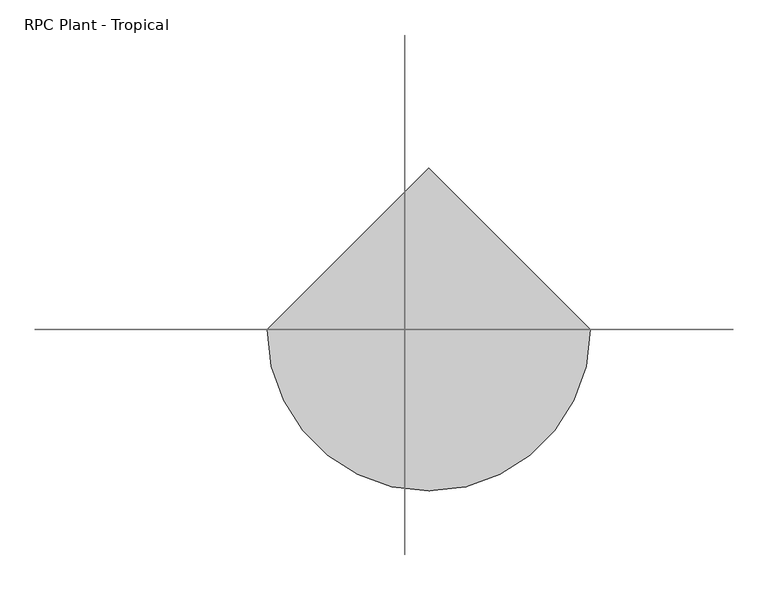
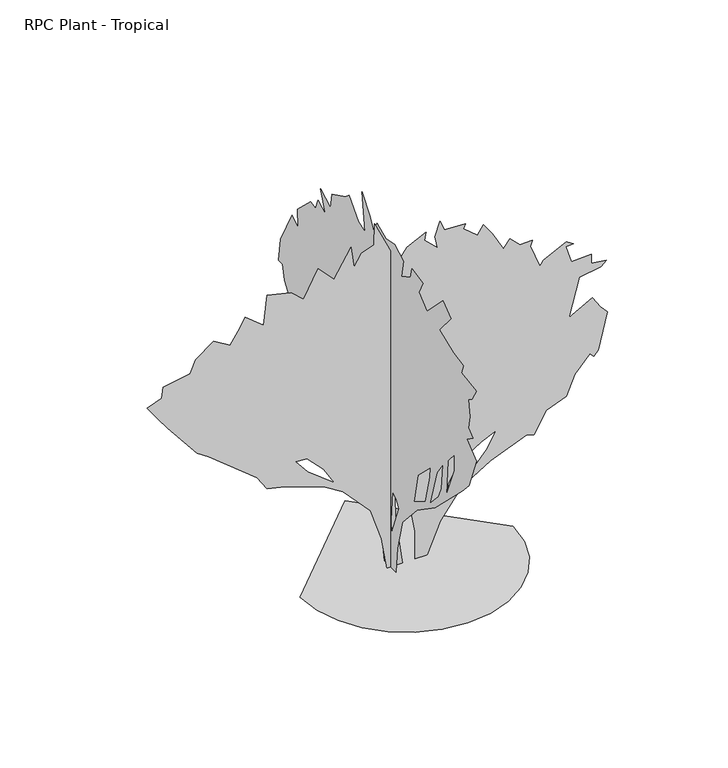
"""IFC4 building model written with IfcOpenShell, lengths in millimetres: geographic element geometry, RPC Plant - Tropical."""

from ifc_helpers import new_model, si_unit, origin, place, context, project, spatial, triangles, source, transform, mapped, element, save


def rpc_plant_tropical_6475341c(model_context):
    return source(origin(), model_context, "Body", "Tessellation", [
        triangles([(-396.3767504, 0.0, 8.22e-05), (-385.8992649, -90.8237077, 8.22e-05), (-356.0543206, -174.2306261, 8.22e-05), (-309.2370838, -247.8313661, 8.22e-05), (-247.8313661, -309.2370838, 8.22e-05), (-174.2306261, -356.0543206, 8.22e-05), (-90.8237077, -385.8992649, 8.22e-05), (1.73e-05, -396.3767504, 8.22e-05), (90.8237077, -385.8992649, 8.22e-05), (174.2306261, -356.0543206, 8.22e-05), (247.8313661, -309.2370838, 8.22e-05), (309.2370838, -247.8313661, 8.22e-05), (356.0543206, -174.2306261, 8.22e-05), (385.8992649, -90.8237077, 8.22e-05), (396.3767504, 3.47e-05, 8.22e-05), (-5.2e-05, 396.3767504, 8.22e-05), (-59.3577095, -35.0059915, 9.26e-05), (-59.3577095, -44.8705806, 101.5460546), (-59.3577095, -75.4742449, 222.0478563), (-59.3577095, -168.9964434, 326.3007588), (-59.3577095, -285.8741748, 405.6706235), (-59.3579639, -459.2340692, 576.3228888), (-59.3579639, -503.9253456, 625.6344137), (-59.3579639, -553.1479589, 751.1941189), (-59.3579639, -491.6190474, 799.7715317), (-59.3579639, -530.478485, 828.915465), (-59.3579639, -501.3320083, 851.5849388), (-59.3579639, -511.0474763, 900.1598808), (-59.3579639, -501.3320083, 961.688756), (-59.3579639, -524.0014821, 977.8812269), (-59.3579639, -553.1479589, 1026.4561689), (-59.3579639, -455.9955677, 1039.4101748), (-59.3579639, -469.4956884, 1077.0376745), (-59.3579639, -404.1821606, 1087.9850441), (-59.3579639, -313.5068087, 1123.6085238), (-59.3579639, -387.9896896, 1211.0454105), (-59.3579639, -336.1762825, 1249.9048119), (-59.3579639, -235.7859349, 1149.5164627), (-59.3579639, -183.9712561, 1191.6144018), (-59.3579639, -209.8784683, 1243.4278816), (-59.3579639, -138.9198272, 1256.3183739), (-59.3579639, -128.9188388, 1217.5224134), (-59.3579639, -70.6279291, 1185.1373989), (-59.3579639, -83.5816624, 1253.143277), (-59.3579639, -25.4436618, 1284.1769932), (-59.3579639, 29.761912, 1272.5743584), (-59.3579639, 86.0073592, 1299.3586246), (-59.3579639, 110.7212849, 1256.3817421), (-59.3579639, 133.3899957, 1298.4822247), (-59.3579639, 185.2039207, 1363.2496376), (-59.3577095, 165.7739475, 1217.5224134), (-59.3577095, 207.8728858, 1230.4738758), (-59.3577095, 266.3644464, 1299.9199276), (-59.3577095, 292.0717617, 1279.0512886), (-59.3577095, 376.2676217, 1236.950806), (-59.3577095, 385.9830897, 1178.660396), (-59.3577095, 450.7505027, 1214.2838757), (-59.3577095, 418.3680679, 1133.3239918), (-59.3577095, 466.9429736, 1159.22946), (-59.3577095, 484.2835213, 1117.1086298), (-59.3577095, 515.5204227, 1123.6085238), (-59.3577095, 599.7162646, 1042.6486399), (-59.3577095, 596.4777632, 974.6427618), (-59.3577095, 635.3397079, 997.3122356), (-59.3577095, 709.8225889, 858.0619417), (-59.3577095, 722.7765947, 767.3865898), (-59.3577095, 696.8686558, 767.3865898), (-59.3577095, 683.91465, 712.3346449), (-59.3577095, 619.147237, 621.659293), (-59.3577095, 586.7622588, 628.1362959), (-59.3577095, 577.0493342, 595.7513177), (-59.3577095, 544.664356, 589.2743148), (-59.3577095, 512.2819213, 514.7914338), (-59.3577095, 453.9890041, 501.8400078), (-59.3577095, 473.4199765, 479.1705339), (-59.3577095, 438.083507, 433.2245012), (-59.3577095, 424.8450708, 430.5955919), (-59.3577095, 359.671251, 388.3935531), (-59.3577095, 230.5626891, 332.9860339), (-59.3577095, 112.6590482, 224.7923109), (-59.3577095, 55.1474106, 87.2636415), (-59.3577095, 39.476642, 8.38e-05), (-59.3577095, -5.8605105, 135.9018064), (-59.3577095, -2.7896791, 186.1833303), (-59.3577095, -12.337225, 304.2967785), (-59.3577095, -38.2442317, 288.1068329), (-59.3577095, -54.4362076, 262.1988576), (-59.3577095, -151.5875587, 349.6357444), (-59.3577095, -177.4947618, 469.4550296), (-59.3577095, -258.4549001, 547.176412), (-59.3577095, -255.2163986, 508.3169744), (-59.3577095, -226.0704487, 394.9721486), (-59.3577095, -255.2163986, 404.687653), (-59.3577095, -297.3143196, 550.4149135), (-59.3577095, -337.517407, 606.5056758), (-59.3577095, -326.4607781, 505.0785092), (-59.3577095, -307.0298058, 462.9780267), (-59.3577095, -358.8432129, 501.8400078), (-59.3579639, -368.5587173, 641.0903017), (-59.3579639, -410.6591635, 689.6651711), (-59.3579639, -410.6591635, 628.1362959), (-59.3577095, 198.157654, 356.112711), (-59.3577095, 261.769596, 391.7057055), (-59.3577095, 324.4541782, 475.9320325), (-59.3577095, 282.3562755, 469.4550296), (-59.3577095, 253.2100531, 430.5955919), (-267.2940953, 2.61e-05, 404.687653), (-308.6096875, 2.21e-05, 471.3142911), (-370.9208914, 1.84e-05, 534.2224425), (-413.0213739, 1.82e-05, 537.4609076), (-368.4215527, 2.15e-05, 482.1804156), (30.6369404, 5.02e-05, 0.0), (31.1304627, 4.38e-05, 108.1619844), (9.0696959, 3.61e-05, 237.4841779), (-47.0839311, 3.05e-05, 330.2047357), (-39.4309189, 4.01e-05, 170.4041154), (-14.7000316, 5.02e-05, 0.0), (-72.990889, 5.02e-05, 0.0), (-92.9872747, 4.29e-05, 122.5858678), (-134.4006626, 3.55e-05, 247.1552083), (-236.0793036, 2.88e-05, 358.7517941), (-302.2063538, 2.64e-05, 398.8659516), (-451.8807753, 2.32e-05, 453.2625587), (-519.8892331, 2.22e-05, 469.4550296), (-555.510133, 1.89e-05, 524.5069382), (-736.858366, 1.03e-05, 670.234235), (-778.9587759, 8.5e-06, 699.3807117), (-889.0625931, 4e-07, 835.3924679), (-924.6860727, -2.5e-06, 883.9674099), (-965.6003632, -6e-06, 942.4685629), (-911.7320669, -7.1e-06, 961.688756), (-905.255064, -9.6e-06, 1003.7892385), (-804.8642441, -1.06e-05, 1019.979166), (-785.4357788, -1.35e-05, 1068.5565788), (-717.4299007, -1.64e-05, 1117.1315208), (-655.8984821, -1.43e-05, 1081.5105846), (-620.2775459, -1.75e-05, 1136.5625296), (-600.8465735, -1.97e-05, 1172.1833931), (-532.8406591, -1.64e-05, 1117.1315208), (-519.8892331, -2.31e-05, 1230.4738758), (-429.2138449, -2.18e-05, 1207.8068727), (-383.8748972, -1.93e-05, 1165.7064629), (-328.8229886, -2.53e-05, 1266.0972828), (-270.5325967, -2.16e-05, 1204.5684076), (-205.7644389, -2.78e-05, 1308.1951492), (-196.0496976, -2.29e-05, 1227.2378815), (-167.6639666, -2.55e-05, 1270.8241745), (-121.5665623, -2.66e-05, 1288.7668293), (-119.7654549, -3.15e-05, 1371.5986919), (-34.1304544, -2.06e-05, 1188.3759367), (2.3015577, -2.34e-05, 1235.4267712), (72.7363851, -2.54e-05, 1269.3357479), (66.2596456, -2.37e-05, 1240.1892712), (114.8353143, -2.1e-05, 1194.8529396), (105.1200825, -2.37e-05, 1240.1892712), (124.5505553, -2.7e-05, 1295.2437595), (140.7425266, -2.47e-05, 1256.3817421), (218.4636638, -2.45e-05, 1253.143277), (211.1367854, -2.35e-05, 1235.7950626), (263.8015941, -2.08e-05, 1191.6144018), (286.4685245, -2.27e-05, 1223.9994164), (318.8535027, -2e-05, 1178.660396), (360.9514054, -1.56e-05, 1104.177515), (385.0814006, -1.75e-05, 1135.7446289), (422.4828604, -1.52e-05, 1097.7005121), (467.8192646, -1.54e-05, 1100.9390499), (461.3422617, -1.41e-05, 1078.2721195), (496.9657413, -8.7e-06, 987.5967676), (509.9172037, -9.8e-06, 1007.0277037), (594.1155527, -1.23e-05, 1049.1256428), (620.0235643, -1.14e-05, 1032.9331718), (593.290058, -1.13e-05, 1031.1069025), (613.5465614, -7.3e-06, 964.9272211), (688.0294424, -7.5e-06, 968.1657589), (688.0294424, -5.4e-06, 932.5448227), (743.0813147, -5e-06, 926.0678198), (723.6503786, -3.8e-06, 906.6368837), (642.6904947, -3.1e-06, 893.6828779), (603.8310571, 5.6e-06, 747.9555811), (691.2679075, 2.7e-06, 796.5330666), (720.4118408, 5.4e-06, 751.1941189), (746.3198524, 7.2e-06, 722.0501856), (713.9348379, 1.55e-05, 582.7973482), (697.7449104, 1.66e-05, 563.3688829), (681.5524395, 1.57e-05, 579.5613902), (626.5005672, 1.93e-05, 518.0299353), (594.1155527, 2.38e-05, 443.5470543), (519.6326717, 2.55e-05, 414.403121), (474.2962675, 3.03e-05, 333.4432371), (448.3882922, 2.98e-05, 343.1587415), (311.7719945, 3.3e-05, 288.0331637), (205.1723602, 3.7e-05, 221.2502851), (125.3034072, 4.32e-05, 117.1220752), (75.9746277, 5.02e-05, 0.0), (30.6369404, 3.34e-05, 281.62983), (43.5909303, 2.72e-05, 385.2566442), (7.9686832, 2.28e-05, 459.7395252), (-30.8919575, 2.45e-05, 430.5955919), (-38.6976243, 2.72e-05, 386.112624), (-2.6646859, 3.14e-05, 315.8842435), (150.4575132, 3.75e-05, 213.6229345), (215.0437962, 3.57e-05, 242.9182394), (296.5269221, 3.01e-05, 337.5199505), (331.8074721, 2.65e-05, 398.2106501), (278.0814637, 2.79e-05, 375.0661689), (195.3344433, 3.11e-05, 320.3901821), (154.7673882, 3.52e-05, 251.8887493)], [[15, 16, 1], [14, 15, 1], [14, 1, 2], [13, 14, 2], [13, 2, 3], [13, 3, 4], [12, 13, 4], [11, 12, 4], [11, 4, 5], [11, 5, 6], [11, 6, 7], [11, 7, 8], [11, 8, 9], [11, 9, 10], [93, 90, 91], [93, 91, 92], [90, 93, 94], [95, 98, 99], [83, 17, 18], [98, 95, 96], [49, 50, 51], [56, 57, 58], [88, 85, 86], [48, 49, 51], [102, 84, 85], [83, 18, 19], [87, 83, 19], [30, 31, 32], [87, 19, 20], [39, 40, 41], [39, 41, 42], [25, 26, 27], [29, 30, 32], [82, 17, 83], [81, 82, 83], [80, 81, 83], [80, 83, 84], [80, 84, 102], [79, 80, 102], [79, 102, 103], [78, 79, 103], [78, 103, 104], [77, 78, 104], [32, 33, 34], [65, 66, 67], [58, 59, 60], [35, 36, 37], [35, 37, 38], [88, 86, 87], [88, 87, 20], [92, 88, 20], [92, 20, 21], [93, 92, 21], [97, 93, 21], [97, 21, 22], [63, 64, 65], [52, 53, 54], [46, 47, 48], [74, 75, 76], [23, 24, 25], [43, 44, 45], [43, 45, 46], [98, 96, 97], [98, 97, 22], [101, 98, 22], [101, 22, 23], [101, 23, 25], [100, 101, 25], [68, 69, 70], [74, 76, 77], [74, 77, 104], [70, 71, 72], [85, 88, 89], [102, 85, 89], [106, 102, 89], [105, 106, 89], [52, 54, 55], [52, 55, 56], [60, 61, 62], [60, 62, 63], [39, 42, 43], [72, 73, 74], [43, 46, 48], [43, 48, 51], [63, 65, 67], [90, 94, 95], [105, 89, 90], [38, 39, 43], [63, 67, 68], [63, 68, 70], [63, 70, 72], [60, 63, 72], [58, 60, 72], [58, 72, 74], [58, 74, 104], [58, 104, 105], [58, 105, 90], [56, 58, 90], [52, 56, 90], [51, 52, 90], [43, 51, 90], [38, 43, 90], [38, 90, 95], [38, 95, 99], [38, 99, 100], [35, 38, 100], [35, 100, 25], [35, 25, 27], [34, 35, 27], [32, 34, 27], [29, 32, 27], [28, 29, 27], [196, 112, 113], [196, 197, 201], [195, 196, 113], [195, 113, 114], [148, 149, 150], [112, 196, 201], [170, 171, 172], [207, 201, 197], [144, 145, 146], [155, 156, 157], [175, 176, 177], [175, 177, 178], [151, 152, 153], [194, 112, 201], [193, 194, 201], [192, 193, 201], [192, 201, 202], [191, 192, 202], [191, 202, 203], [195, 114, 115], [200, 195, 115], [199, 200, 115], [169, 170, 172], [206, 207, 197], [157, 158, 159], [165, 166, 167], [160, 161, 162], [142, 143, 144], [129, 130, 131], [116, 117, 118], [116, 118, 119], [116, 119, 120], [115, 116, 120], [107, 115, 120], [107, 120, 121], [107, 121, 122], [111, 107, 122], [111, 122, 123], [110, 111, 123], [137, 138, 139], [199, 115, 107], [163, 164, 165], [139, 140, 141], [183, 184, 185], [190, 191, 203], [190, 203, 204], [173, 174, 175], [173, 175, 178], [169, 172, 173], [179, 180, 181], [198, 199, 107], [139, 141, 142], [188, 189, 190], [110, 123, 124], [110, 124, 125], [168, 169, 173], [154, 155, 157], [154, 157, 159], [131, 132, 133], [182, 183, 185], [188, 190, 204], [147, 148, 150], [146, 147, 150], [205, 206, 197], [136, 137, 139], [181, 182, 185], [179, 181, 185], [179, 185, 186], [134, 135, 136], [198, 107, 108], [154, 159, 160], [133, 134, 136], [168, 173, 178], [168, 178, 179], [129, 131, 133], [128, 129, 133], [127, 128, 133], [127, 133, 136], [126, 127, 136], [126, 136, 139], [125, 126, 139], [110, 125, 139], [110, 139, 142], [109, 110, 142], [109, 142, 144], [109, 144, 146], [109, 146, 150], [108, 109, 150], [198, 108, 150], [197, 198, 150], [205, 197, 150], [204, 205, 150], [188, 204, 150], [187, 188, 150], [186, 187, 150], [179, 186, 150], [168, 179, 150], [167, 168, 150], [150, 151, 153], [150, 153, 154], [160, 162, 163], [154, 160, 163], [150, 154, 163], [167, 150, 163], [167, 163, 165]], closed=False),
    ])


if __name__ == "__main__":
    model = new_model("IFC4")
    model_context = context("Model", 3, world=origin())
    ifc_project = project(units=[si_unit("LENGTHUNIT", "METRE", prefix="MILLI")], contexts=[model_context])
    site = spatial("IfcSite", under=ifc_project)
    building = spatial("IfcBuilding", under=site)
    placement = place(None, origin())
    rpc_plant_tropical_shape = rpc_plant_tropical_6475341c(model_context)
    element("IfcGeographicElement", 1, ObjectType="RPC Plant - Tropical", at=placement, inside=building, context=model_context, shape_type="MappedRepresentation", body=[
        mapped(rpc_plant_tropical_shape, transform((0.0, 0.0, 0.0), x_axis=(1.0, 0.0, 0.0), y_axis=(0.0, 1.0, 0.0), z_axis=(0.0, 0.0, 1.0))),
    ])
    save(model, "model.ifc")

# Revit data of these elements
# Type "RPC Plant - Tropical"
#   built-in parameter 1005198 = "{2, 15},{39, RPC-16-G3GK-N2Q0-PN0G-6000-ST1L-LVER-AU},{1, 0},{1, 0},{2, 13},{1, 8},{5, Color},{1, 0},{1, 0},{3, 0.8},{3, 0.8},{3, 0.8},{1, 8},{7, BBoxMin},{1, 0},{1, 0},{1, 0},{1, 0},{1, 0},{1, 8},{7, BBoxMax},{1, 0},{1, 0},{1, 0},{1, 0},{1, 0},{2, 11},{9, RPCTypeId},{1, 0},{1, 0},{39, RPC-16-G3GK-N2Q0-PN0G-6000-ST1L-LVER-AU},{1, 6},{14, RPCPlantHeight},{1, 0},{1, 0},{3, 4.5},{2, 11},{7, keyword},{1, 0},{1, 0},{35, :RPCs:Shrubs [General]:Geometry:RPC},{2, 11},{8, category},{1, 0},{1, 0},{16, Shrubs [General]},{2, 11},{12, LocalizedUID},{1, 0},{1, 0},{12, Honey Myrtle},{2, 14},{6, Height},{1, 0},{1, 0},{3, 4.5},{1, 2},{16, Cast Reflections},{1, 0},{1, 0},{1, 0},{1, 2},{12, Cast Shadows},{1, 0},{1, 0},{1, 1},{1, 2},{9, Lock View},{1, 0},{1, 0},{1, 0},{1, 4},{5, ViewC},{1, 0},{1, 0},{1, 0},{21, assetlibrary_base.fbx},{1, 5},"
#   built-in parameter 1005195 = "RPC-16-G3GK-N2Q0-PN0G-6000-ST1L-LVER-AU"
#   Assembly Code = "G2050500"
#   Height = 4' - 6"
#   Default Elevation = 0
